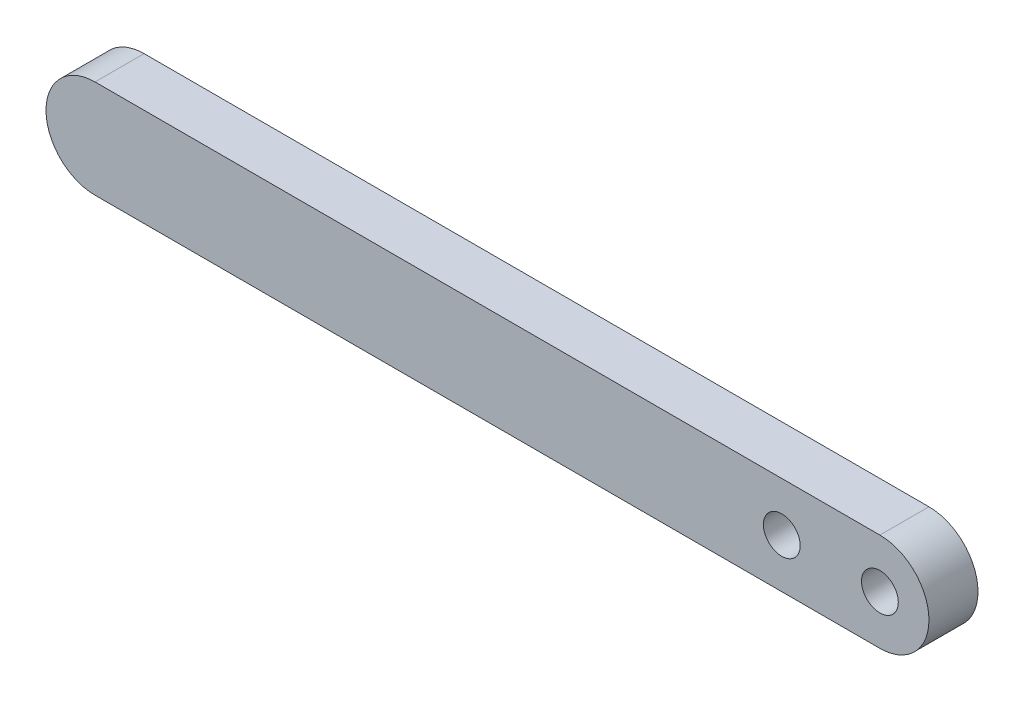
from build123d import *

# Parameters (mm, degrees)
HANDLE_PROFILE_SKETCH_R        = 0.09375
HANDLE_BAR_EXTRUDE_DEPTH       = 0.125
SCALE_X25_4_TO_INCH_SIZE_SCALE = 25.4


with BuildPart() as part:
    # Handle Profile Sketch → Handle Bar Extrude (new, symmetric)
    with BuildSketch(Plane.XY):
        with BuildLine():
            Line((-2, 0.25), (2, 0.25))
            ThreePointArc((2, 0.25), (2.25, 0), (2, -0.25))
            Line((2, -0.25), (-2, -0.25))
            ThreePointArc((-2, -0.25), (-2.25, 0), (-2, 0.25))
        make_face()
        with Locations((2, 0)):
            Circle(HANDLE_PROFILE_SKETCH_R, mode=Mode.SUBTRACT)
        with Locations((1.5, 0)):
            Circle(HANDLE_PROFILE_SKETCH_R, mode=Mode.SUBTRACT)
    extrude(amount=HANDLE_BAR_EXTRUDE_DEPTH, both=True)


with BuildPart() as part_1:
    # Scale x25.4 to Inch Size: scaled about (0, 0, 0)
    add(part.part.scale(SCALE_X25_4_TO_INCH_SIZE_SCALE))


solid = part_1.part
